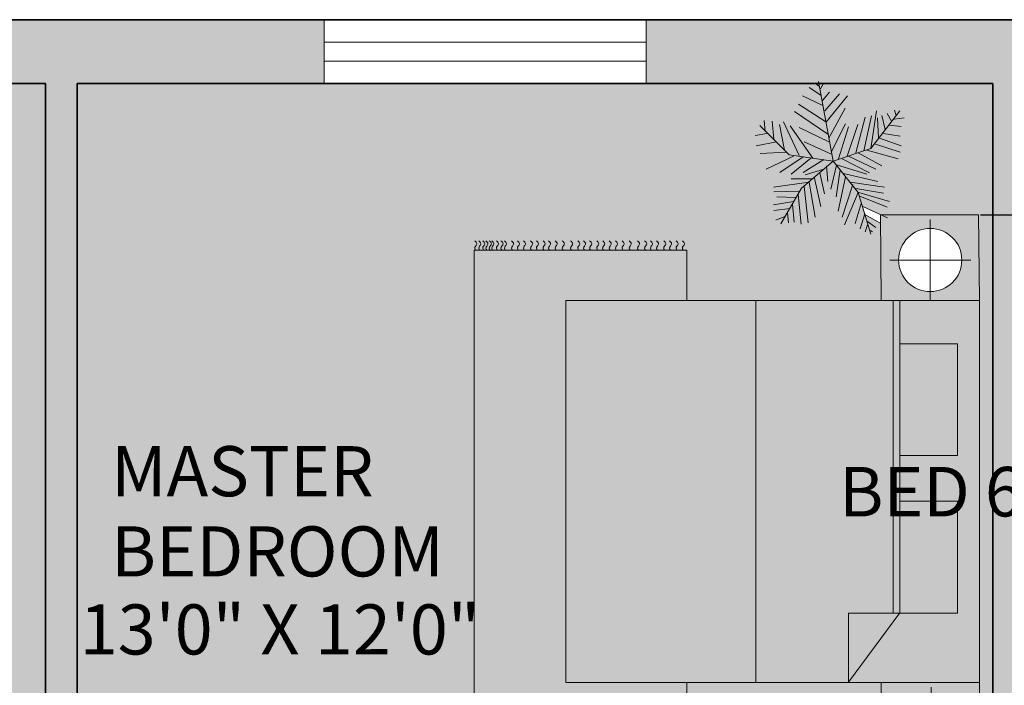
# Model space of a CAD drawing. Units: inches. Extents: x 1316 to 1777, y 813 to 1650.
# Tile 20 of 22: x 1567 to 1706, y 1481 to 1575. Entities that reach past the tile are written whole.
import ezdxf

# ---------------------------------------------------------------- set-up
doc = ezdxf.new("R2010")
doc.units = ezdxf.units.IN
doc.header["$MEASUREMENT"] = 0
for name, color, linetype, lineweight in [('A-ANNO-DIMS', 2, 'Continuous', 18), ('A-AREA-IDEN', 7, 'Continuous', 18), ('A-FURN-PATT', 23, 'Continuous', 13), ('A-WALL-PATT', 250, 'Continuous', 13), ('furniture', 23, 'Continuous', 18), ('greenary', 106, 'Continuous', 13), ('walls', 250, 'Continuous', 35), ('windows', 141, 'Continuous', 18)]:
    doc.layers.add(name, color=color, linetype=linetype, lineweight=lineweight)
doc.layers.add('A-FLOR-PATT', color=254, linetype='Continuous', lineweight=13, true_color=0xfeeab9)
doc.styles.get("Standard").update_dxf_attribs({"font": 'arial.ttf'})
doc.dimstyles.get("Standard").update_dxf_attribs({"dimtxt": 7, "dimasz": 0.18, "dimexe": 0.18, "dimexo": 0.0625, "dimgap": 0.09, "dimtad": 0, "dimtih": 1, "dimtoh": 1, "dimzin": 0, "dimdsep": 46, "dimlunit": 3, "dimtxsty": 'Standard', "dimcen": 0.09, "dimadec": 0, "dimazin": 0, "dimtfac": 1, "dimtofl": 0, "dimtmove": 0, "dimatfit": 3, "dimfxl": 1, "dimtolj": 1, "dimtzin": 0, "dimarcsym": 0})

# ---------------------------------------------------------------- blocks, each defined once
blk = doc.blocks.new('*U13')
for p, q in [((0, 0), (-10.5, 57)), ((-8.737, 47.138), (-17.069, 52.711)), ((-10.186, 53.64), (-13.084, 55.962)), ((-9.099, 51.782), (-6.563, 55.962)), ((-7.65, 43.423), (-2.578, 49.46)), ((-7.288, 39.707), (-21.778, 46.673)), ((-5.839, 35.992), (4.667, 48.067)), ((-5.114, 27.632), (10.463, 46.673)), ((-3.665, 19.273), (-27.574, 35.527)), ((-5.114, 28.097), (-24.676, 40.636)), ((-2.941, 16.486), (8.652, 37.85)), ((27, 9), (48, 36)), ((27.127, 9.056), (31.112, 35.992)), ((44.153, 36.456), (45.239, 32.741)), ((-48.585, 21.131), (-49.309, 29.026)), ((-43.513, 28.561), (-42.427, 15.558)), ((16.259, 5.805), (23.142, 31.348)), ((22.055, 7.198), (27.489, 32.277)), ((31.836, 30.883), (32.561, 16.486)), ((35.096, 32.741), (37.27, 22.524)), ((38.719, 34.134), (41.979, 28.561)), ((43.791, 29.954), (51.036, 30.883)), ((-31.5, 4.5), (-52.5, 25.5)), ((-38.442, 26.239), (-34.819, 7.663)), ((-35.544, 28.097), (-24.314, 3.947)), ((-14.533, 2.09), (-30.834, 25.31)), ((-24.314, 23.917), (-2.941, 13.7)), ((-1.129, 6.734), (9.014, 26.704)), ((3.942, 1.625), (11.187, 24.381)), ((10.101, 3.483), (17.708, 26.239)), ((40.53, 25.775), (48.862, 24.846)), ((-47.498, 19.737), (-55.83, 18.344)), ((33.285, 16.486), (48.862, 10.913)), ((36.183, 19.737), (48.137, 17.88)), ((-40.615, 13.7), (-55.105, 10.913)), ((-20.691, 13.7), (-1.129, 4.876)), ((0, 0), (27, 9)), ((24.229, 7.663), (46.688, 1.625)), ((29.662, 12.307), (48.137, 6.269)), ((-33.37, 6.269), (-52.207, 5.34)), ((-28.299, 3.483), (-47.86, -5.805)), ((-21.416, 3.018), (-38.079, -8.128)), ((0, 0), (-31.5, 4.5)), ((-15.982, 2.09), (-30.11, -9.521)), ((0, 0), (-22.5, -19.5)), ((-6.563, 1.161), (-21.416, -8.128)), ((0, 0), (18, -22.5)), ((6.478, 1.625), (26.04, -8.592)), ((11.187, 3.483), (30.749, -5.805)), ((18.07, 5.805), (35.096, -3.483)), ((-6.563, -5.805), (-19.967, -9.985)), ((-4.752, -3.483), (-3.665, -14.629)), ((2.493, -3.019), (-1.491, -20.202)), ((1.769, -2.555), (24.229, -9.521)), ((5.029, -6.27), (2.131, -25.775)), ((-15.257, -12.772), (-30.11, -12.772)), ((-13.446, -11.378), (-8.737, -32.741)), ((-9.461, -8.592), (-6.201, -23.453)), ((9.014, -11.378), (3.58, -35.992)), ((7.565, -9.056), (32.198, -14.629)), ((-17.431, -15.094), (-42.789, -18.809)), ((-22.5, -19.5), (-37.5, -45)), ((-20.691, -18.345), (-17.793, -44.352)), ((-17.069, -15.094), (-12.721, -40.172)), ((14.085, -16.951), (6.478, -40.172)), ((12.274, -15.094), (36.907, -18.809)), ((16.259, -19.738), (36.183, -22.989)), ((-24.314, -21.596), (-42.427, -22.06)), ((-26.849, -26.24), (-40.253, -25.775)), ((-25.038, -23.918), (-22.865, -45.281)), ((18.07, -22.524), (8.289, -45.745)), ((18, -22.5), (27, -52.5)), ((18.433, -22.524), (40.53, -29.026)), ((19.157, -25.311), (38.719, -33.206)), ((-28.299, -29.026), (-42.789, -31.348)), ((-30.834, -34.135), (-42.427, -35.528)), ((-29.023, -30.884), (-27.936, -43.887)), ((20.244, -30.419), (15.897, -44.816)), ((21.331, -32.741), (39.081, -40.636)), ((-34.457, -39.708), (-40.978, -42.494)), ((-32.646, -36.921), (-31.921, -44.352)), ((22.78, -37.85), (19.519, -48.532)), ((22.78, -38.314), (34.372, -44.816)), ((24.591, -45.745), (23.142, -50.854)), ((24.591, -43.423), (30.749, -47.603)), ((26.764, -49.925), (28.213, -50.854))]:
    blk.add_line(p, q)
blk = doc.blocks.new('CARPET')
at = {"layer": 'furniture'}
for p, q in [((-51.53, -98.11), (-51.53, -55.12)), ((-51.53, -55.12), (-41.27, -55.12)), ((36, -55.12), (51.55, -55.12)), ((51.55, -55.12), (51.55, -98.11)), ((51.55, -98.11), (-51.53, -98.11))]:
    blk.add_line(p, q, dxfattribs=at)
for points, knots in [([(-53.37, -55.99), (-53.22, -55.8), (-52.9, -55.41), (-52.34, -55.8), (-51.89, -56.08), (-51.65, -55.91), (-51.53, -55.83)], [0, 0, 0, 0, 0.653278, 1.290138, 1.740457, 2.114451, 2.114451, 2.114451, 2.114451]), ([(53.37, -55.99), (53.22, -55.8), (52.9, -55.41), (52.34, -55.8), (51.89, -56.08), (51.65, -55.91), (51.53, -55.83)], [0, 0, 0, 0, 0.653278, 1.290138, 1.740457, 2.114451, 2.114451, 2.114451, 2.114451]), ([(-53.37, -57.26), (-53.22, -57.07), (-52.9, -56.67), (-52.34, -57.07), (-51.89, -57.35), (-51.65, -57.17), (-51.53, -57.1)], [0, 0, 0, 0, 0.653278, 1.290138, 1.740457, 2.114451, 2.114451, 2.114451, 2.114451]), ([(53.37, -57.26), (53.22, -57.07), (52.9, -56.67), (52.34, -57.07), (51.89, -57.35), (51.65, -57.17), (51.53, -57.1)], [0, 0, 0, 0, 0.653278, 1.290138, 1.740457, 2.114451, 2.114451, 2.114451, 2.114451]), ([(-53.37, -58.59), (-53.22, -58.4), (-52.9, -58.01), (-52.34, -58.4), (-51.89, -58.68), (-51.65, -58.5), (-51.53, -58.43)], [0, 0, 0, 0, 0.653278, 1.290138, 1.740457, 2.114451, 2.114451, 2.114451, 2.114451]), ([(-53.37, -59.78), (-53.22, -59.58), (-52.9, -59.19), (-52.34, -59.58), (-51.89, -59.86), (-51.65, -59.69), (-51.53, -59.61)], [0, 0, 0, 0, 0.653278, 1.290138, 1.740457, 2.114451, 2.114451, 2.114451, 2.114451]), ([(53.37, -58.59), (53.22, -58.4), (52.9, -58.01), (52.34, -58.4), (51.89, -58.68), (51.65, -58.5), (51.53, -58.43)], [0, 0, 0, 0, 0.653278, 1.290138, 1.740457, 2.114451, 2.114451, 2.114451, 2.114451]), ([(53.37, -59.78), (53.22, -59.58), (52.9, -59.19), (52.34, -59.58), (51.89, -59.86), (51.65, -59.69), (51.53, -59.61)], [0, 0, 0, 0, 0.653278, 1.290138, 1.740457, 2.114451, 2.114451, 2.114451, 2.114451]), ([(-53.37, -61.22), (-53.22, -61.02), (-52.9, -60.63), (-52.34, -61.02), (-51.89, -61.3), (-51.65, -61.13), (-51.53, -61.05)], [0, 0, 0, 0, 0.653278, 1.290138, 1.740457, 2.114451, 2.114451, 2.114451, 2.114451]), ([(53.37, -61.22), (53.22, -61.02), (52.9, -60.63), (52.34, -61.02), (51.89, -61.3), (51.65, -61.13), (51.53, -61.05)], [0, 0, 0, 0, 0.653278, 1.290138, 1.740457, 2.114451, 2.114451, 2.114451, 2.114451]), ([(-53.37, -62.44), (-53.22, -62.25), (-52.9, -61.86), (-52.34, -62.25), (-51.89, -62.53), (-51.65, -62.36), (-51.53, -62.28)], [0, 0, 0, 0, 0.653278, 1.290138, 1.740457, 2.114451, 2.114451, 2.114451, 2.114451]), ([(-53.37, -63.63), (-53.22, -63.43), (-52.9, -63.04), (-52.34, -63.43), (-51.89, -63.72), (-51.65, -63.54), (-51.53, -63.46)], [0, 0, 0, 0, 0.653278, 1.290138, 1.740457, 2.114451, 2.114451, 2.114451, 2.114451]), ([(53.37, -62.44), (53.22, -62.25), (52.9, -61.86), (52.34, -62.25), (51.89, -62.53), (51.65, -62.36), (51.53, -62.28)], [0, 0, 0, 0, 0.653278, 1.290138, 1.740457, 2.114451, 2.114451, 2.114451, 2.114451]), ([(53.37, -63.63), (53.22, -63.43), (52.9, -63.04), (52.34, -63.43), (51.89, -63.72), (51.65, -63.54), (51.53, -63.46)], [0, 0, 0, 0, 0.653278, 1.290138, 1.740457, 2.114451, 2.114451, 2.114451, 2.114451]), ([(-53.37, -65.07), (-53.22, -64.87), (-52.9, -64.48), (-52.34, -64.87), (-51.89, -65.15), (-51.65, -64.98), (-51.53, -64.9)], [0, 0, 0, 0, 0.653278, 1.290138, 1.740457, 2.114451, 2.114451, 2.114451, 2.114451]), ([(53.37, -65.07), (53.22, -64.87), (52.9, -64.48), (52.34, -64.87), (51.89, -65.15), (51.65, -64.98), (51.53, -64.9)], [0, 0, 0, 0, 0.653278, 1.290138, 1.740457, 2.114451, 2.114451, 2.114451, 2.114451]), ([(-53.37, -66.76), (-53.22, -66.56), (-52.9, -66.17), (-52.34, -66.56), (-51.89, -66.84), (-51.65, -66.67), (-51.53, -66.59)], [0, 0, 0, 0, 0.653278, 1.290138, 1.740457, 2.114451, 2.114451, 2.114451, 2.114451]), ([(53.37, -66.76), (53.22, -66.56), (52.9, -66.17), (52.34, -66.56), (51.89, -66.84), (51.65, -66.67), (51.53, -66.59)], [0, 0, 0, 0, 0.653278, 1.290138, 1.740457, 2.114451, 2.114451, 2.114451, 2.114451]), ([(-53.37, -68.2), (-53.22, -68), (-52.9, -67.61), (-52.34, -68), (-51.89, -68.28), (-51.65, -68.11), (-51.53, -68.03)], [0, 0, 0, 0, 0.653278, 1.290138, 1.740457, 2.114451, 2.114451, 2.114451, 2.114451]), ([(-53.37, -69.53), (-53.22, -69.33), (-52.9, -68.94), (-52.34, -69.33), (-51.89, -69.61), (-51.65, -69.44), (-51.53, -69.36)], [0, 0, 0, 0, 0.653278, 1.290138, 1.740457, 2.114451, 2.114451, 2.114451, 2.114451]), ([(53.37, -68.2), (53.22, -68), (52.9, -67.61), (52.34, -68), (51.89, -68.28), (51.65, -68.11), (51.53, -68.03)], [0, 0, 0, 0, 0.653278, 1.290138, 1.740457, 2.114451, 2.114451, 2.114451, 2.114451]), ([(53.37, -69.53), (53.22, -69.33), (52.9, -68.94), (52.34, -69.33), (51.89, -69.61), (51.65, -69.44), (51.53, -69.36)], [0, 0, 0, 0, 0.653278, 1.290138, 1.740457, 2.114451, 2.114451, 2.114451, 2.114451]), ([(-53.37, -70.79), (-53.22, -70.6), (-52.9, -70.21), (-52.34, -70.6), (-51.89, -70.88), (-51.65, -70.7), (-51.53, -70.63)], [0, 0, 0, 0, 0.653278, 1.290138, 1.740457, 2.114451, 2.114451, 2.114451, 2.114451]), ([(-53.37, -72.12), (-53.22, -71.93), (-52.9, -71.54), (-52.34, -71.93), (-51.89, -72.21), (-51.65, -72.04), (-51.53, -71.96)], [0, 0, 0, 0, 0.653278, 1.290138, 1.740457, 2.114451, 2.114451, 2.114451, 2.114451]), ([(53.37, -70.79), (53.22, -70.6), (52.9, -70.21), (52.34, -70.6), (51.89, -70.88), (51.65, -70.7), (51.53, -70.63)], [0, 0, 0, 0, 0.653278, 1.290138, 1.740457, 2.114451, 2.114451, 2.114451, 2.114451]), ([(53.37, -72.12), (53.22, -71.93), (52.9, -71.54), (52.34, -71.93), (51.89, -72.21), (51.65, -72.04), (51.53, -71.96)], [0, 0, 0, 0, 0.653278, 1.290138, 1.740457, 2.114451, 2.114451, 2.114451, 2.114451]), ([(-53.37, -73.31), (-53.22, -73.11), (-52.9, -72.72), (-52.34, -73.11), (-51.89, -73.4), (-51.65, -73.22), (-51.53, -73.14)], [0, 0, 0, 0, 0.653278, 1.290138, 1.740457, 2.114451, 2.114451, 2.114451, 2.114451]), ([(53.37, -73.31), (53.22, -73.11), (52.9, -72.72), (52.34, -73.11), (51.89, -73.4), (51.65, -73.22), (51.53, -73.14)], [0, 0, 0, 0, 0.653278, 1.290138, 1.740457, 2.114451, 2.114451, 2.114451, 2.114451]), ([(-53.37, -74.75), (-53.22, -74.55), (-52.9, -74.16), (-52.34, -74.55), (-51.89, -74.83), (-51.65, -74.66), (-51.53, -74.58)], [0, 0, 0, 0, 0.653278, 1.290138, 1.740457, 2.114451, 2.114451, 2.114451, 2.114451]), ([(-53.37, -75.98), (-53.22, -75.78), (-52.9, -75.39), (-52.34, -75.78), (-51.89, -76.06), (-51.65, -75.89), (-51.53, -75.81)], [0, 0, 0, 0, 0.653278, 1.290138, 1.740457, 2.114451, 2.114451, 2.114451, 2.114451]), ([(53.37, -74.75), (53.22, -74.55), (52.9, -74.16), (52.34, -74.55), (51.89, -74.83), (51.65, -74.66), (51.53, -74.58)], [0, 0, 0, 0, 0.653278, 1.290138, 1.740457, 2.114451, 2.114451, 2.114451, 2.114451]), ([(53.37, -75.98), (53.22, -75.78), (52.9, -75.39), (52.34, -75.78), (51.89, -76.06), (51.65, -75.89), (51.53, -75.81)], [0, 0, 0, 0, 0.653278, 1.290138, 1.740457, 2.114451, 2.114451, 2.114451, 2.114451]), ([(-53.37, -77.16), (-53.22, -76.96), (-52.9, -76.57), (-52.34, -76.96), (-51.89, -77.25), (-51.65, -77.07), (-51.53, -76.99)], [0, 0, 0, 0, 0.653278, 1.290138, 1.740457, 2.114451, 2.114451, 2.114451, 2.114451]), ([(53.37, -77.16), (53.22, -76.96), (52.9, -76.57), (52.34, -76.96), (51.89, -77.25), (51.65, -77.07), (51.53, -76.99)], [0, 0, 0, 0, 0.653278, 1.290138, 1.740457, 2.114451, 2.114451, 2.114451, 2.114451]), ([(-53.37, -78.6), (-53.22, -78.4), (-52.9, -78.01), (-52.34, -78.4), (-51.89, -78.68), (-51.65, -78.51), (-51.53, -78.43)], [0, 0, 0, 0, 0.653278, 1.290138, 1.740457, 2.114451, 2.114451, 2.114451, 2.114451]), ([(53.37, -78.6), (53.22, -78.4), (52.9, -78.01), (52.34, -78.4), (51.89, -78.68), (51.65, -78.51), (51.53, -78.43)], [0, 0, 0, 0, 0.653278, 1.290138, 1.740457, 2.114451, 2.114451, 2.114451, 2.114451]), ([(-53.37, -80.29), (-53.22, -80.09), (-52.9, -79.7), (-52.34, -80.09), (-51.89, -80.37), (-51.65, -80.2), (-51.53, -80.12)], [0, 0, 0, 0, 0.653278, 1.290138, 1.740457, 2.114451, 2.114451, 2.114451, 2.114451]), ([(-53.37, -81.73), (-53.22, -81.53), (-52.9, -81.14), (-52.34, -81.53), (-51.89, -81.81), (-51.65, -81.64), (-51.53, -81.56)], [0, 0, 0, 0, 0.653278, 1.290138, 1.740457, 2.114451, 2.114451, 2.114451, 2.114451]), ([(53.37, -80.29), (53.22, -80.09), (52.9, -79.7), (52.34, -80.09), (51.89, -80.37), (51.65, -80.2), (51.53, -80.12)], [0, 0, 0, 0, 0.653278, 1.290138, 1.740457, 2.114451, 2.114451, 2.114451, 2.114451]), ([(53.37, -81.73), (53.22, -81.53), (52.9, -81.14), (52.34, -81.53), (51.89, -81.81), (51.65, -81.64), (51.53, -81.56)], [0, 0, 0, 0, 0.653278, 1.290138, 1.740457, 2.114451, 2.114451, 2.114451, 2.114451]), ([(-53.37, -83.06), (-53.22, -82.86), (-52.9, -82.47), (-52.34, -82.86), (-51.89, -83.14), (-51.65, -82.97), (-51.53, -82.89)], [0, 0, 0, 0, 0.653278, 1.290138, 1.740457, 2.114451, 2.114451, 2.114451, 2.114451]), ([(53.37, -83.06), (53.22, -82.86), (52.9, -82.47), (52.34, -82.86), (51.89, -83.14), (51.65, -82.97), (51.53, -82.89)], [0, 0, 0, 0, 0.653278, 1.290138, 1.740457, 2.114451, 2.114451, 2.114451, 2.114451]), ([(-53.37, -84.18), (-53.22, -83.99), (-52.9, -83.6), (-52.34, -83.99), (-51.89, -84.27), (-51.65, -84.09), (-51.53, -84.02)], [0, 0, 0, 0, 0.653278, 1.290138, 1.740457, 2.114451, 2.114451, 2.114451, 2.114451]), ([(-53.37, -85.51), (-53.22, -85.32), (-52.9, -84.93), (-52.34, -85.32), (-51.89, -85.6), (-51.65, -85.42), (-51.53, -85.35)], [0, 0, 0, 0, 0.653278, 1.290138, 1.740457, 2.114451, 2.114451, 2.114451, 2.114451]), ([(53.37, -84.18), (53.22, -83.99), (52.9, -83.6), (52.34, -83.99), (51.89, -84.27), (51.65, -84.09), (51.53, -84.02)], [0, 0, 0, 0, 0.653278, 1.290138, 1.740457, 2.114451, 2.114451, 2.114451, 2.114451]), ([(53.37, -85.51), (53.22, -85.32), (52.9, -84.93), (52.34, -85.32), (51.89, -85.6), (51.65, -85.42), (51.53, -85.35)], [0, 0, 0, 0, 0.653278, 1.290138, 1.740457, 2.114451, 2.114451, 2.114451, 2.114451]), ([(-53.37, -86.7), (-53.22, -86.5), (-52.9, -86.11), (-52.34, -86.5), (-51.89, -86.78), (-51.65, -86.61), (-51.53, -86.53)], [0, 0, 0, 0, 0.653278, 1.290138, 1.740457, 2.114451, 2.114451, 2.114451, 2.114451]), ([(53.37, -86.7), (53.22, -86.5), (52.9, -86.11), (52.34, -86.5), (51.89, -86.78), (51.65, -86.61), (51.53, -86.53)], [0, 0, 0, 0, 0.653278, 1.290138, 1.740457, 2.114451, 2.114451, 2.114451, 2.114451]), ([(-53.37, -88.14), (-53.22, -87.94), (-52.9, -87.55), (-52.34, -87.94), (-51.89, -88.22), (-51.65, -88.05), (-51.53, -87.97)], [0, 0, 0, 0, 0.653278, 1.290138, 1.740457, 2.114451, 2.114451, 2.114451, 2.114451]), ([(-53.37, -89.36), (-53.22, -89.17), (-52.9, -88.78), (-52.34, -89.17), (-51.89, -89.45), (-51.65, -89.28), (-51.53, -89.2)], [0, 0, 0, 0, 0.653278, 1.290138, 1.740457, 2.114451, 2.114451, 2.114451, 2.114451]), ([(53.37, -88.14), (53.22, -87.94), (52.9, -87.55), (52.34, -87.94), (51.89, -88.22), (51.65, -88.05), (51.53, -87.97)], [0, 0, 0, 0, 0.653278, 1.290138, 1.740457, 2.114451, 2.114451, 2.114451, 2.114451]), ([(53.37, -89.36), (53.22, -89.17), (52.9, -88.78), (52.34, -89.17), (51.89, -89.45), (51.65, -89.28), (51.53, -89.2)], [0, 0, 0, 0, 0.653278, 1.290138, 1.740457, 2.114451, 2.114451, 2.114451, 2.114451]), ([(-53.37, -90.55), (-53.22, -90.35), (-52.9, -89.96), (-52.34, -90.35), (-51.89, -90.64), (-51.65, -90.46), (-51.53, -90.38)], [0, 0, 0, 0, 0.653278, 1.290138, 1.740457, 2.114451, 2.114451, 2.114451, 2.114451]), ([(-53.37, -91.99), (-53.22, -91.79), (-52.9, -91.4), (-52.34, -91.79), (-51.89, -92.07), (-51.65, -91.9), (-51.53, -91.82)], [0, 0, 0, 0, 0.653278, 1.290138, 1.740457, 2.114451, 2.114451, 2.114451, 2.114451]), ([(53.37, -90.55), (53.22, -90.35), (52.9, -89.96), (52.34, -90.35), (51.9, -90.63), (51.66, -90.47), (51.55, -90.4)], [0, 0, 0, 0, 0.653278, 1.290138, 1.740457, 2.0926, 2.0926, 2.0926, 2.0926]), ([(53.37, -91.99), (53.22, -91.79), (52.9, -91.4), (52.34, -91.79), (51.9, -92.07), (51.66, -91.91), (51.55, -91.83)], [0, 0, 0, 0, 0.653278, 1.290138, 1.740457, 2.0926, 2.0926, 2.0926, 2.0926]), ([(-53.37, -92.69), (-53.22, -92.48), (-52.9, -92.08), (-52.35, -92.49), (-51.89, -92.77), (-51.65, -92.6), (-51.53, -92.52)], [0, 0, 0, 0, 0.663904, 1.307406, 1.757725, 2.131719, 2.131719, 2.131719, 2.131719]), ([(-53.37, -93.61), (-53.22, -93.42), (-52.9, -93.03), (-52.34, -93.42), (-51.89, -93.7), (-51.65, -93.52), (-51.53, -93.45)], [0, 0, 0, 0, 0.653278, 1.290138, 1.740457, 2.114451, 2.114451, 2.114451, 2.114451]), ([(53.37, -92.69), (53.22, -92.49), (52.9, -92.09), (52.34, -92.49), (51.9, -92.77), (51.66, -92.61), (51.55, -92.53)], [0, 0, 0, 0, 0.656792, 1.295826, 1.746145, 2.098292, 2.098292, 2.098292, 2.098292]), ([(53.37, -93.66), (53.22, -93.46), (52.9, -93.07), (52.34, -93.46), (51.9, -93.74), (51.66, -93.58), (51.55, -93.5)], [0, 0, 0, 0, 0.653278, 1.290138, 1.740457, 2.0926, 2.0926, 2.0926, 2.0926]), ([(-53.37, -94.55), (-53.22, -94.35), (-52.9, -93.96), (-52.34, -94.35), (-51.89, -94.63), (-51.65, -94.46), (-51.53, -94.38)], [0, 0, 0, 0, 0.653278, 1.290138, 1.740457, 2.114451, 2.114451, 2.114451, 2.114451]), ([(-53.37, -95.05), (-53.22, -94.85), (-52.9, -94.46), (-52.34, -94.85), (-51.89, -95.14), (-51.65, -94.96), (-51.53, -94.88)], [0, 0, 0, 0, 0.653278, 1.290138, 1.740457, 2.114451, 2.114451, 2.114451, 2.114451]), ([(-53.37, -95.73), (-53.22, -95.54), (-52.9, -95.15), (-52.34, -95.54), (-51.89, -95.82), (-51.65, -95.65), (-51.53, -95.57)], [0, 0, 0, 0, 0.653278, 1.290138, 1.740457, 2.114451, 2.114451, 2.114451, 2.114451]), ([(53.37, -95.78), (53.22, -95.58), (52.9, -95.19), (52.34, -95.58), (51.89, -95.86), (51.65, -95.69), (51.53, -95.61)], [0, 0, 0, 0, 0.653278, 1.290138, 1.740457, 2.114451, 2.114451, 2.114451, 2.114451]), ([(53.37, -94.59), (53.22, -94.4), (52.9, -94.01), (52.34, -94.4), (51.9, -94.68), (51.66, -94.51), (51.55, -94.44)], [0, 0, 0, 0, 0.653278, 1.290138, 1.740457, 2.0926, 2.0926, 2.0926, 2.0926]), ([(53.37, -95.1), (53.22, -94.9), (52.9, -94.51), (52.34, -94.9), (51.9, -95.18), (51.66, -95.02), (51.55, -94.94)], [0, 0, 0, 0, 0.653278, 1.290138, 1.740457, 2.0926, 2.0926, 2.0926, 2.0926]), ([(-53.37, -96.38), (-53.22, -96.18), (-52.9, -95.79), (-52.34, -96.18), (-51.89, -96.47), (-51.65, -96.29), (-51.53, -96.21)], [0, 0, 0, 0, 0.653278, 1.290138, 1.740457, 2.114451, 2.114451, 2.114451, 2.114451]), ([(-53.37, -97.17), (-53.22, -96.98), (-52.9, -96.59), (-52.34, -96.98), (-51.89, -97.26), (-51.65, -97.08), (-51.53, -97.01)], [0, 0, 0, 0, 0.653278, 1.290138, 1.740457, 2.114451, 2.114451, 2.114451, 2.114451]), ([(-53.37, -97.99), (-53.22, -97.79), (-52.9, -97.4), (-52.34, -97.79), (-51.89, -98.08), (-51.65, -97.9), (-51.53, -97.82)], [0, 0, 0, 0, 0.653278, 1.290138, 1.740457, 2.114451, 2.114451, 2.114451, 2.114451]), ([(53.37, -96.43), (53.22, -96.23), (52.9, -95.84), (52.34, -96.23), (51.89, -96.51), (51.65, -96.34), (51.53, -96.26)], [0, 0, 0, 0, 0.653278, 1.290138, 1.740457, 2.114451, 2.114451, 2.114451, 2.114451]), ([(53.37, -97.22), (53.22, -97.02), (52.9, -96.63), (52.34, -97.02), (51.89, -97.3), (51.65, -97.13), (51.53, -97.05)], [0, 0, 0, 0, 0.653278, 1.290138, 1.740457, 2.114451, 2.114451, 2.114451, 2.114451]), ([(53.37, -97.99), (53.22, -97.79), (52.9, -97.4), (52.34, -97.79), (51.89, -98.08), (51.65, -97.9), (51.53, -97.82)], [0, 0, 0, 0, 0.653278, 1.290138, 1.740457, 2.114451, 2.114451, 2.114451, 2.114451])]:
    blk.add_open_spline(points, degree=3, knots=knots, dxfattribs=at)
blk = doc.blocks.new('A$C58D270C6')
at = {"layer": 'furniture'}
for p, q in [((9.09, 124.13), (9.09, 108.87)), ((1.46, 116.5), (16.73, 116.5)), ((14.97, 94.84), (24.62, 107.92)), ((24.62, 94.93), (24.62, 107.92)), ((42.08, 108), (42.08, 36)), ((14.97, 94.93), (24.62, 94.93)), ((14.97, 94.84), (14.97, 36)), ((16.22, 94.93), (16.22, 36)), ((9.25, 36), (9.25, 20.74)), ((1.62, 28.37), (16.88, 28.37))]:
    blk.add_line(p, q, dxfattribs=at)
for points in [[(18.5, 108), (18.34, 124.13), (-0.16, 124.13), (0, 108)], [(0, 108), (77.91, 108), (77.91, 36), (0, 36)], [(4.09, 94.93), (14.97, 94.93), (14.97, 73.83), (4.09, 73.83)], [(4.09, 65.23), (14.97, 65.23), (14.97, 44.13), (4.09, 44.13)], [(18.65, 19.87), (18.5, 36), (0, 36), (0.16, 19.87)]]:
    blk.add_lwpolyline(points, close=True, dxfattribs=at)
for centre in [(9.09, 116.5), (9.25, 28.37)]:
    blk.add_circle(centre, 5.95, dxfattribs=at)
at = {"layer": 'furniture', "xscale": 0.9312884925094044, "yscale": 0.9312884925094044, "zscale": 0.9312884925094044, "rotation": 90}
blk.add_blockref('CARPET', (3.79, 74.47), dxfattribs=at)
blk = doc.blocks.new('WINDOW-45_5x9')
for p, q in [((0, 9), (0, 0)), ((45.51, 9), (0, 9)), ((45.51, 0), (45.51, 9)), ((0, 5.82), (45.51, 5.82)), ((45.51, 5.82), (45.51, 3.15)), ((45.51, 3.15), (0, 3.15)), ((0, 0), (45.51, 0))]:
    blk.add_line(p, q)
blk = doc.blocks.new('*D28')
at = {"layer": 'A-ANNO-DIMS', "color": 0, "lineweight": -2, "transparency": 16777216}
for p, q in [((1702.47, 1547.78), (1714.32, 1547.78)), ((1714.14, 1547.6), (1714.14, 1512.32)), ((1714.14, 1469.72), (1714.14, 1504.99)), ((1702.47, 1469.54), (1714.32, 1469.54))]:
    blk.add_line(p, q, dxfattribs=at)
at = {"layer": 'A-ANNO-DIMS', "color": 0, "transparency": 16777216}
for points in [[(1714.11, 1547.6), (1714.17, 1547.6), (1714.14, 1547.78)], [(1714.11, 1469.72), (1714.17, 1469.72), (1714.14, 1469.54)]]:
    blk.add_solid(points, dxfattribs=at)
at = {"layer": 'Defpoints', "color": 0, "transparency": 16777216}
for p in [(1702.41, 1547.78), (1702.41, 1469.54), (1714.14, 1469.54)]:
    blk.add_point(p, dxfattribs=at)
at = {"layer": 'A-ANNO-DIMS', "color": 0, "transparency": 16777216, "insert": (1714.14, 1508.66), "char_height": 7, "attachment_point": 5}
blk.add_mtext('\\A1;BED 6\'-6" TYP.', dxfattribs=at)

msp = doc.modelspace()

# ---------------------------------------------------------------- hatches: boundary and pattern name
at = {"layer": 'A-FLOR-PATT'}
h = msp.add_hatch(color=256, dxfattribs=at)
h.dxf.hatch_style = 1
h.paths.add_polyline_path([(1704.173, 1566.369), (1574.845, 1566.369), (1574.845, 1434.369), (1704.173, 1434.369)])
h.paths.add_polyline_path([(1630.932, 1542.856), (1660.956, 1542.856), (1660.956, 1535.716), (1688.427, 1535.716), (1688.322, 1546.604), (1686.085, 1547.859), (1686.091, 1547.88), (1685.166, 1550.963), (1681.619, 1555.397), (1678.246, 1552.474), (1678.253, 1552.433), (1678.187, 1552.423), (1681.619, 1555.397), (1683.601, 1556.058), (1683.639, 1556.172), (1683.764, 1556.112), (1686.94, 1557.171), (1688.039, 1558.585), (1688.034, 1558.699), (1688.108, 1558.672), (1686.969, 1557.208), (1686.965, 1557.18), (1681.619, 1555.397), (1682.039, 1554.872), (1682.12, 1554.846), (1682.107, 1554.788), (1685.145, 1550.989), (1685.188, 1550.977), (1685.173, 1550.941), (1685.764, 1548.971), (1688.364, 1547.814), (1702.185, 1547.814), (1702.301, 1535.716), (1702.301, 1481.716), (1702.418, 1469.617), (1688.544, 1469.617), (1688.427, 1481.716), (1660.956, 1481.716), (1660.956, 1470.853), (1630.932, 1470.853)], flags=16)
h.paths.add_polyline_path([(1624.931, 1450.279), (1703.919, 1450.279), (1703.919, 1436.32), (1703.919, 1435.026), (1624.931, 1435.026), (1624.931, 1435.469)], flags=16)
h.paths.add_polyline_path([(1624.931, 1443.714), (1625.995, 1443.714), (1625.995, 1449.229), (1626.752, 1449.229), (1626.752, 1443.714), (1628.114, 1443.714), (1628.114, 1449.229), (1628.871, 1449.229), (1628.871, 1443.714), (1630.502, 1443.714), (1630.502, 1449.229), (1631.259, 1449.229), (1631.259, 1443.714), (1632.968, 1443.714), (1632.968, 1449.229), (1633.724, 1449.229), (1633.724, 1443.714), (1638.318, 1443.714), (1641.013, 1449.6), (1641.689, 1449.29), (1639.136, 1443.714), (1640.128, 1443.714), (1642.823, 1449.6), (1643.499, 1449.29), (1640.945, 1443.714), (1642.323, 1443.714), (1645.018, 1449.6), (1645.694, 1449.29), (1643.141, 1443.714), (1647.035, 1443.714), (1647.035, 1449.229), (1647.792, 1449.229), (1647.792, 1443.714), (1649.606, 1443.714), (1649.606, 1449.229), (1650.363, 1449.229), (1650.363, 1443.714), (1652.865, 1443.714), (1652.865, 1449.229), (1653.621, 1449.229), (1653.621, 1443.714), (1657.035, 1443.714), (1657.035, 1449.229), (1657.792, 1449.229), (1657.792, 1443.714), (1660.083, 1443.714), (1660.083, 1449.229), (1660.839, 1449.229), (1660.839, 1443.714), (1662.605, 1443.714), (1662.605, 1449.229), (1663.362, 1449.229), (1663.362, 1443.714), (1667.702, 1443.714), (1667.702, 1449.229), (1668.459, 1449.229), (1668.459, 1443.714), (1671.655, 1443.714), (1670.316, 1449.229), (1671.051, 1449.407), (1672.434, 1443.714), (1679.696, 1443.714), (1680.179, 1449.244), (1680.933, 1449.178), (1680.455, 1443.714), (1683.5, 1443.714), (1682.225, 1448.723), (1682.959, 1448.91), (1684.281, 1443.714), (1688.219, 1443.714), (1688.219, 1449.229), (1688.976, 1449.229), (1688.976, 1443.714), (1690.482, 1443.714), (1690.482, 1449.229), (1691.239, 1449.229), (1691.239, 1443.714), (1692.488, 1443.714), (1692.488, 1449.229), (1693.245, 1449.229), (1693.245, 1443.714), (1695.009, 1443.714), (1695.009, 1449.229), (1695.766, 1449.229), (1695.766, 1443.714), (1701.029, 1443.714), (1700.875, 1443.379), (1695.766, 1443.379), (1695.766, 1435.872), (1695.009, 1435.872), (1695.009, 1443.379), (1693.245, 1443.379), (1693.245, 1435.872), (1692.488, 1435.872), (1692.488, 1443.379), (1691.239, 1443.379), (1691.239, 1435.872), (1690.482, 1435.872), (1690.482, 1443.379), (1688.976, 1443.379), (1688.976, 1435.872), (1688.219, 1435.872), (1688.219, 1443.379), (1684.366, 1443.379), (1686.252, 1435.965), (1685.518, 1435.779), (1683.585, 1443.379), (1680.426, 1443.379), (1679.77, 1435.872), (1679.016, 1435.938), (1679.666, 1443.379), (1677.602, 1443.379), (1677.602, 1435.46), (1676.845, 1435.46), (1676.845, 1443.379), (1672.515, 1443.379), (1674.202, 1436.427), (1673.467, 1436.249), (1671.736, 1443.379), (1668.459, 1443.379), (1668.459, 1435.872), (1667.702, 1435.872), (1667.702, 1443.379), (1663.362, 1443.379), (1663.362, 1435.872), (1662.605, 1435.872), (1662.605, 1443.379), (1660.839, 1443.379), (1660.839, 1435.872), (1660.083, 1435.872), (1660.083, 1443.379), (1657.792, 1443.379), (1657.792, 1435.872), (1657.035, 1435.872), (1657.035, 1443.379), (1653.621, 1443.379), (1653.621, 1435.872), (1652.865, 1435.872), (1652.865, 1443.379), (1650.363, 1443.379), (1650.363, 1435.872), (1649.606, 1435.872), (1649.606, 1443.379), (1647.792, 1443.379), (1647.792, 1435.872), (1647.035, 1435.872), (1647.035, 1443.379), (1642.988, 1443.379), (1639.39, 1435.522), (1638.715, 1435.832), (1642.17, 1443.379), (1640.792, 1443.379), (1637.195, 1435.522), (1636.519, 1435.832), (1639.974, 1443.379), (1638.983, 1443.379), (1635.385, 1435.522), (1634.709, 1435.832), (1638.165, 1443.379), (1633.724, 1443.379), (1633.724, 1435.872), (1632.968, 1435.872), (1632.968, 1443.379), (1631.259, 1443.379), (1631.259, 1435.872), (1630.502, 1435.872), (1630.502, 1443.379), (1628.871, 1443.379), (1628.871, 1435.872), (1628.114, 1435.872), (1628.114, 1443.379), (1626.752, 1443.379), (1626.752, 1435.872), (1625.995, 1435.872), (1625.995, 1443.379), (1624.931, 1443.379)], flags=0)
h.paths.add_polyline_path([(1683.839, 1491.517), (1691.022, 1491.517), (1691.071, 1491.582), (1691.071, 1529.618), (1699.231, 1529.618), (1699.231, 1513.795), (1691.071, 1513.795), (1691.071, 1507.34), (1699.231, 1507.34), (1699.231, 1491.517), (1691.022, 1491.517), (1683.839, 1481.774)], flags=0)
h.paths.add_polyline_path([(1691.015, 1475.341, -1), (1699.947, 1475.341, -1)], flags=0)
h.paths.add_polyline_path([(1690.898, 1541.439, -1), (1699.83, 1541.439, -1)], flags=0)
h.paths.add_polyline_path([(1505.845, 1469.591), (1505.845, 1566.369), (1386.064, 1566.369), (1386.064, 1450.329), (1465.697, 1450.329), (1465.697, 1449.245), (1466.177, 1449.025), (1465.697, 1447.977), (1465.697, 1436.055), (1465.697, 1434.369), (1505.845, 1434.369), (1505.845, 1440.551), (1476.949, 1440.551), (1476.949, 1441.822), (1476.977, 1441.822, -0.4000145)])
edge = h.paths.add_edge_path(flags=16)
edge.add_spline(control_points=[(1456.973, 1471.794), (1457.023, 1471.721), (1457.138, 1471.554), (1456.942, 1471.242), (1456.67, 1470.851), (1456.943, 1470.632), (1457.081, 1470.522)], knot_values=[0, 0, 0, 0, 0.3521435, 0.8024629, 1.4393222, 2.0926005, 2.0926005, 2.0926005, 2.0926005], degree=3, periodic=0)
edge.add_spline(control_points=[(1457.325, 1471.794), (1457.375, 1471.721), (1457.49, 1471.554), (1457.294, 1471.242), (1457.022, 1470.851), (1457.295, 1470.632), (1457.433, 1470.522)], knot_values=[0, 0, 0, 0, 0.3521435, 0.8024629, 1.4393222, 2.0926005, 2.0926005, 2.0926005, 2.0926005], degree=3, periodic=0)
edge = h.paths.add_edge_path(flags=16)
edge.add_line((1429.513, 1471.794), (1429.513, 1482.657))
edge.add_line((1429.513, 1482.657), (1402.042, 1482.657))
edge.add_line((1402.042, 1482.657), (1401.925, 1470.559))
edge.add_line((1401.925, 1470.559), (1388.051, 1470.559))
edge.add_line((1388.051, 1470.559), (1388.167, 1482.657))
edge.add_line((1388.167, 1482.657), (1388.167, 1536.657))
edge.add_line((1388.167, 1536.657), (1388.284, 1548.755))
edge.add_line((1388.284, 1548.755), (1402.158, 1548.755))
edge.add_line((1402.158, 1548.755), (1402.042, 1536.657))
edge.add_line((1402.042, 1536.657), (1429.513, 1536.657))
edge.add_line((1429.513, 1536.657), (1429.513, 1543.797))
edge.add_line((1429.513, 1543.797), (1456.932, 1543.797))
edge.add_spline(control_points=[(1456.932, 1543.797), (1456.987, 1543.874), (1457.108, 1544.044), (1456.911, 1544.361), (1456.638, 1544.752), (1456.911, 1544.971), (1457.049, 1545.082)], knot_values=[0, 0, 0, 0, 0.3739943, 0.8243137, 1.461173, 2.1144513, 2.1144513, 2.1144513, 2.1144513], degree=3, periodic=0)
edge.add_spline(control_points=[(1457.401, 1545.082), (1457.263, 1544.971), (1456.99, 1544.752), (1457.263, 1544.361), (1457.46, 1544.044), (1457.339, 1543.874), (1457.284, 1543.797)], knot_values=[0, 0, 0, 0, 0.6532783, 1.2901376, 1.740457, 2.1144513, 2.1144513, 2.1144513, 2.1144513], degree=3, periodic=0)
edge.add_line((1457.284, 1543.797), (1459.536, 1543.797))
edge.add_line((1459.536, 1543.797), (1459.536, 1471.794))
edge.add_line((1459.536, 1471.794), (1429.513, 1471.794))
h.paths.add_polyline_path([(1406.63, 1482.715), (1399.446, 1492.458), (1399.398, 1492.458), (1391.238, 1492.458), (1391.238, 1508.281), (1399.398, 1508.281), (1399.398, 1514.736), (1391.238, 1514.736), (1391.238, 1530.559), (1399.398, 1530.559), (1399.398, 1492.524), (1399.446, 1492.458), (1406.63, 1492.458)], flags=0)
h.paths.add_polyline_path([(1399.454, 1476.282, -1), (1390.522, 1476.282, -1)], flags=0)
h.paths.add_polyline_path([(1390.638, 1542.38, -1), (1399.571, 1542.38, -1)], flags=0)
h.paths.add_polyline_path([(1487.293, 1548.286), (1487.08, 1548.252), (1487.104, 1547.964)], flags=16)
h.paths.add_polyline_path([(1491.493, 1552.843), (1490.887, 1552.654), (1490.949, 1552.372)], flags=16)
h.paths.add_polyline_path([(1489.966, 1554.409), (1489.859, 1554.561), (1489.718, 1554.445)], flags=16)
h.paths.add_polyline_path([(1497.301, 1546.483), (1497.294, 1546.462), (1497.309, 1546.453)], flags=16)
h.paths.add_polyline_path([(1496.386, 1549.553), (1492.828, 1554), (1492.655, 1554.939), (1492.454, 1555.029), (1492.589, 1555.296), (1491.806, 1559.547), (1491.869, 1559.506), (1491.824, 1559.451), (1492.828, 1554), (1494.81, 1554.661), (1494.848, 1554.774), (1494.973, 1554.715), (1496.01, 1555.061), (1496.078, 1555.314), (1496.341, 1555.171), (1498.15, 1555.774), (1499.249, 1557.187), (1499.243, 1557.301), (1499.317, 1557.275), (1498.179, 1555.811), (1498.174, 1555.782), (1492.828, 1554), (1493.249, 1553.474), (1493.33, 1553.449), (1493.316, 1553.39), (1495.203, 1551.032), (1495.702, 1550.957), (1495.574, 1550.568), (1496.354, 1549.592), (1496.397, 1549.58)], flags=16)
h.paths.add_polyline_path([(1486.021, 1555.224), (1485.958, 1555.549), (1483.595, 1557.912), (1483.28, 1557.859), (1483.243, 1558.264), (1486.27, 1555.237)], flags=16)
h.paths.add_polyline_path([(1505.845, 1469.591, 0.4000145), (1476.977, 1441.822), (1505.845, 1441.822)], flags=17)
h = msp.add_hatch(color=256, dxfattribs=at)
h.dxf.hatch_style = 1
h.paths.add_polyline_path([(1561.016, 1510.243), (1561.016, 1510.275), (1562.477, 1510.275), (1562.477, 1476.879), (1562.477, 1471.869), (1529.081, 1471.869), (1529.081, 1476.879, -0.4014527)])
h.paths.add_polyline_path([(1570.345, 1566.369), (1510.345, 1566.369), (1510.345, 1502.159), (1526.605, 1502.159), (1526.605, 1480.004), (1510.345, 1480.004), (1510.345, 1476.369), (1529.081, 1476.369), (1529.081, 1476.879, -0.4014527), (1561.016, 1510.243), (1561.016, 1510.275), (1562.477, 1510.275), (1562.477, 1476.369), (1570.345, 1476.369)])
h.paths.add_polyline_path([(1528.659, 1540.982), (1528.659, 1542.825), (1529.12, 1552.041), (1528.659, 1552.041), (1528.659, 1553.884), (1529.12, 1553.884, -0.206081), (1535.571, 1559.041), (1535.571, 1561.257), (1534.65, 1561.257), (1534.65, 1562.179), (1532.806, 1562.179), (1532.806, 1563.1), (1543.866, 1563.1), (1543.866, 1562.179), (1542.023, 1562.179), (1542.023, 1561.257), (1541.101, 1561.257), (1541.101, 1559.041, -0.206081), (1547.552, 1553.884), (1548.013, 1553.884), (1548.013, 1552.041), (1547.552, 1552.041), (1547.552, 1542.825), (1548.013, 1542.825), (1548.013, 1540.982)], flags=16)
h.paths.add_polyline_path([(1704.173, 1429.869), (1602.173, 1429.869), (1602.173, 1408.281), (1631.07, 1408.281), (1631.07, 1407.011), (1631.042, 1407.011, -0.4000145), (1602.173, 1379.241), (1602.173, 1369.869), (1625.31, 1369.869), (1625.31, 1385.783), (1647.465, 1385.783), (1647.465, 1369.869), (1704.173, 1369.869)])
h.paths.add_polyline_path([(1669.737, 1382.593), (1670.237, 1382.593), (1670.237, 1392.593), (1669.737, 1392.593), (1669.737, 1394.593), (1690.737, 1394.593), (1690.737, 1392.593), (1690.237, 1392.593), (1690.237, 1382.593), (1690.737, 1382.593), (1690.737, 1380.593), (1690.237, 1380.593, -0.206081), (1683.237, 1374.997), (1683.237, 1372.593), (1684.237, 1372.593), (1684.237, 1371.593), (1686.237, 1371.593), (1686.237, 1370.593), (1674.237, 1370.593), (1674.237, 1371.593), (1676.237, 1371.593), (1676.237, 1372.593), (1677.237, 1372.593), (1677.237, 1374.997, -0.206081), (1670.237, 1380.593), (1669.737, 1380.593)], flags=16)
h.paths.add_polyline_path([(1631.042, 1407.011), (1602.029, 1407.011), (1602.029, 1408.281), (1597.673, 1408.281), (1597.673, 1379.241), (1602.029, 1379.241, 0.4014527)])
at = {"layer": 'A-FURN-PATT'}
h = msp.add_hatch(color=256, dxfattribs=at)
h.dxf.hatch_style = 1
h.paths.add_polyline_path([(1688.416, 1481.677), (1702.29, 1481.677), (1702.407, 1469.579), (1695.469, 1469.579), (1695.469, 1470.836, 0.4142136), (1699.936, 1475.302, 1), (1691.003, 1475.302, 0.4142136), (1695.469, 1470.836), (1695.469, 1469.579), (1688.532, 1469.579)])
h.paths.add_polyline_path([(1691.011, 1491.478), (1699.219, 1491.478), (1699.219, 1507.301), (1691.059, 1507.301), (1691.059, 1513.757), (1699.219, 1513.757), (1699.219, 1529.579), (1691.059, 1529.579), (1691.059, 1535.677), (1702.29, 1535.677), (1702.29, 1481.677), (1683.827, 1481.677), (1683.827, 1481.735)])
h.paths.add_polyline_path([(1690.887, 1541.4, 0.4142136), (1695.353, 1536.934), (1695.353, 1535.677), (1688.416, 1535.677), (1688.299, 1547.775), (1702.173, 1547.775), (1702.29, 1535.677), (1695.353, 1535.677), (1695.353, 1536.934, 0.4142136), (1699.819, 1541.4, 1)])
h = msp.add_hatch(color=256, dxfattribs=at)
h.dxf.hatch_style = 1
h.paths.add_polyline_path([(1691.059, 1507.301), (1699.219, 1507.301), (1699.219, 1491.478), (1691.059, 1491.478)])
h.paths.add_polyline_path([(1691.059, 1529.579), (1699.219, 1529.579), (1699.219, 1513.757), (1691.059, 1513.757)])
h.paths.add_polyline_path([(1630.921, 1542.817), (1660.945, 1542.817), (1660.945, 1535.677), (1643.861, 1535.677), (1643.861, 1481.677), (1660.945, 1481.677), (1660.945, 1470.814), (1630.921, 1470.814)])
h = msp.add_hatch(color=256, dxfattribs=at)
h.dxf.hatch_style = 1
h.paths.add_polyline_path([(1643.861, 1535.677), (1670.731, 1535.677), (1670.731, 1481.677), (1643.861, 1481.677)])
h.paths.add_polyline_path([(1670.731, 1535.677), (1690.127, 1535.677), (1690.127, 1491.478), (1683.827, 1491.478), (1683.827, 1481.677), (1670.731, 1481.677)])
h = msp.add_hatch(color=256, dxfattribs=at)
h.dxf.hatch_style = 1
h.paths.add_polyline_path([(1683.827, 1491.478), (1691.011, 1491.478), (1683.827, 1481.735)])
h.paths.add_polyline_path([(1690.127, 1535.677), (1691.059, 1535.677), (1691.059, 1491.544), (1691.011, 1491.478), (1690.127, 1491.478)])
at = {"layer": 'A-WALL-PATT'}
h = msp.add_hatch(color=256, dxfattribs=at)
h.dxf.hatch_style = 1
h.paths.add_polyline_path([(1713.173, 1281.369), (1656.173, 1281.369), (1656.173, 1298.258), (1651.673, 1298.258), (1651.673, 1281.369), (1567.673, 1281.369), (1567.673, 1266.995), (1572.173, 1266.995), (1572.173, 1276.869), (1704.173, 1276.869), (1704.173, 1132.869), (1608.64, 1132.869), (1608.64, 1123.869), (1704.173, 1123.869), (1704.173, 1040.173), (1652.869, 1040.173), (1652.869, 1031.173), (1713.173, 1031.173), (1713.173, 1040.173)])
h.paths.add_polyline_path([(1572.173, 1237.955), (1567.673, 1237.955), (1567.673, 1123.869), (1583.146, 1123.869), (1583.146, 1132.869), (1572.173, 1132.869)], flags=17)
h.paths.add_polyline_path([(1510.345, 1566.369), (1524.171, 1566.369), (1524.171, 1571.985), (1524.171, 1575.369), (1445.955, 1575.369), (1445.955, 1566.369), (1505.845, 1566.369), (1505.845, 1469.591), (1510.345, 1469.591), (1510.345, 1471.869), (1529.081, 1471.869), (1529.081, 1476.369), (1510.345, 1476.369)])
h.paths.add_polyline_path([(1609.722, 1575.369), (1545.119, 1575.369), (1545.119, 1566.369), (1570.345, 1566.369), (1570.345, 1476.369), (1562.477, 1476.369), (1562.477, 1471.869), (1570.345, 1471.869), (1570.345, 1469.591), (1574.845, 1469.591), (1574.845, 1566.369), (1609.722, 1566.369)])
h.paths.add_polyline_path([(1713.173, 1575.369), (1655.233, 1575.369), (1655.233, 1566.369), (1704.173, 1566.369), (1704.173, 1434.369), (1574.845, 1434.369), (1574.845, 1440.551), (1574.701, 1440.551), (1570.345, 1440.551), (1570.345, 1429.869), (1597.673, 1429.869), (1597.673, 1408.281), (1602.173, 1408.281), (1602.173, 1429.869), (1704.173, 1429.869), (1704.173, 1410.704), (1707.375, 1410.704), (1713.173, 1410.704)])
h.paths.add_polyline_path([(1713.173, 1383.676), (1704.173, 1383.676), (1704.173, 1369.869), (1602.173, 1369.869), (1602.173, 1379.241), (1597.673, 1379.241), (1597.673, 1365.369), (1713.173, 1365.369)])
h.paths.add_polyline_path([(1444.564, 1429.869), (1510.345, 1429.869), (1510.345, 1440.551), (1505.845, 1440.551), (1505.845, 1434.369), (1386.064, 1434.369), (1386.064, 1566.369), (1400.445, 1566.369), (1400.445, 1575.369), (1377.064, 1575.369), (1377.064, 1412.813), (1380.509, 1412.813), (1386.064, 1412.813), (1386.064, 1429.869), (1440.064, 1429.869), (1440.064, 1401.229), (1444.564, 1401.229)])
h.paths.add_polyline_path([(1444.564, 1372.189), (1440.064, 1372.189), (1440.064, 1369.869), (1386.064, 1369.869), (1386.064, 1378.758), (1377.064, 1378.758), (1377.064, 1349.201), (1381.118, 1349.201), (1386.064, 1349.201), (1386.064, 1365.369), (1440.064, 1365.369), (1440.064, 1322.882), (1444.564, 1322.882)])
h.paths.add_polyline_path([(1510.564, 1295.094), (1506.064, 1295.094), (1506.064, 1245.369), (1386.064, 1245.369), (1386.064, 1272.582), (1377.064, 1272.582), (1377.064, 1212.905), (1380.1, 1212.905), (1386.064, 1212.905), (1386.064, 1240.869), (1510.564, 1240.869)])
h.paths.add_polyline_path([(1386.064, 1163.761), (1377.064, 1163.761), (1377.064, 1063.869), (1419.363, 1063.869), (1419.363, 1072.869), (1386.064, 1072.869)])
h.paths.add_polyline_path([(1510.564, 1072.869), (1469.381, 1072.869), (1469.381, 1063.869), (1501.564, 1063.869), (1501.564, 1033.023), (1501.564, 1031.173), (1540.829, 1031.173), (1540.829, 1036.182, -0.0299535), (1541.068, 1040.173), (1510.564, 1040.173)])
h.paths.add_polyline_path([(1607.369, 1040.173), (1574.225, 1040.173), (1574.225, 1036.182), (1574.225, 1031.173), (1607.369, 1031.173)], flags=17)
h.paths.add_polyline_path([(1637.054, 1040.173), (1624.706, 1040.173), (1624.706, 1031.173), (1637.054, 1031.173)], flags=17)

# ---------------------------------------------------------------- linework, layer by layer
at = {"layer": 'walls'}
for p, q in [((1377.064, 1575.369), (1713.173, 1575.369)), ((1510.345, 1566.369), (1570.345, 1566.369)), ((1570.345, 1566.369), (1570.345, 1476.369)), ((1574.845, 1566.369), (1574.845, 1434.369)), ((1574.845, 1566.369), (1704.173, 1566.369)), ((1704.173, 1566.369), (1704.173, 1434.369))]:
    msp.add_line(p, q, dxfattribs=at)

# ---------------------------------------------------------------- block references
at = {"layer": 'furniture', "xscale": 0.7500000390647866, "yscale": 0.7500000390647866, "zscale": 0.7500000390647866, "rotation": 180}
msp.add_blockref('A$C58D270C6', (1702.29, 1562.677), dxfattribs=at)
at = {"layer": 'greenary', "xscale": 0.1970946241996355, "yscale": 0.1970946241996355, "zscale": 0.1970946241996355}
msp.add_blockref('*U13', (1681.619, 1555.397), dxfattribs=at)
at = {"layer": 'windows'}
msp.add_blockref('WINDOW-45_5x9', (1609.723, 1566.369), dxfattribs=at)

# ---------------------------------------------------------------- texts
at = {"layer": 'A-AREA-IDEN'}
for s, height, p in [('MASTER', 7.0829, (1579.623, 1508.012)), ('BEDROOM', 7.0829, (1579.623, 1496.677)), ('13\'0" X 12\'0"', 7.08291, (1575.199, 1485.651))]:
    msp.add_text(s, height=height, dxfattribs=at).set_placement(p)

# ---------------------------------------------------------------- dimensions: what is measured, and where the dimension line sits
at = {"layer": 'A-ANNO-DIMS'}
dim = msp.add_linear_dim(base=(1714.142, 1469.542), p1=(1702.407, 1547.775), p2=(1702.407, 1469.542), angle=270, text='BED <> TYP.', dimstyle='Standard', override={"dimdec": 1, "dimlfac": 1, "dimrnd": 0, "dimzin": 1, "dimdsep": 46, "dimlunit": 4, "dimfrac": 2}, dxfattribs=at)
dim.commit()
dim.dimension.update_dxf_attribs({"geometry": '*D28', "text_midpoint": (1714.142, 1508.658)})

doc.saveas('drawing.dxf')
